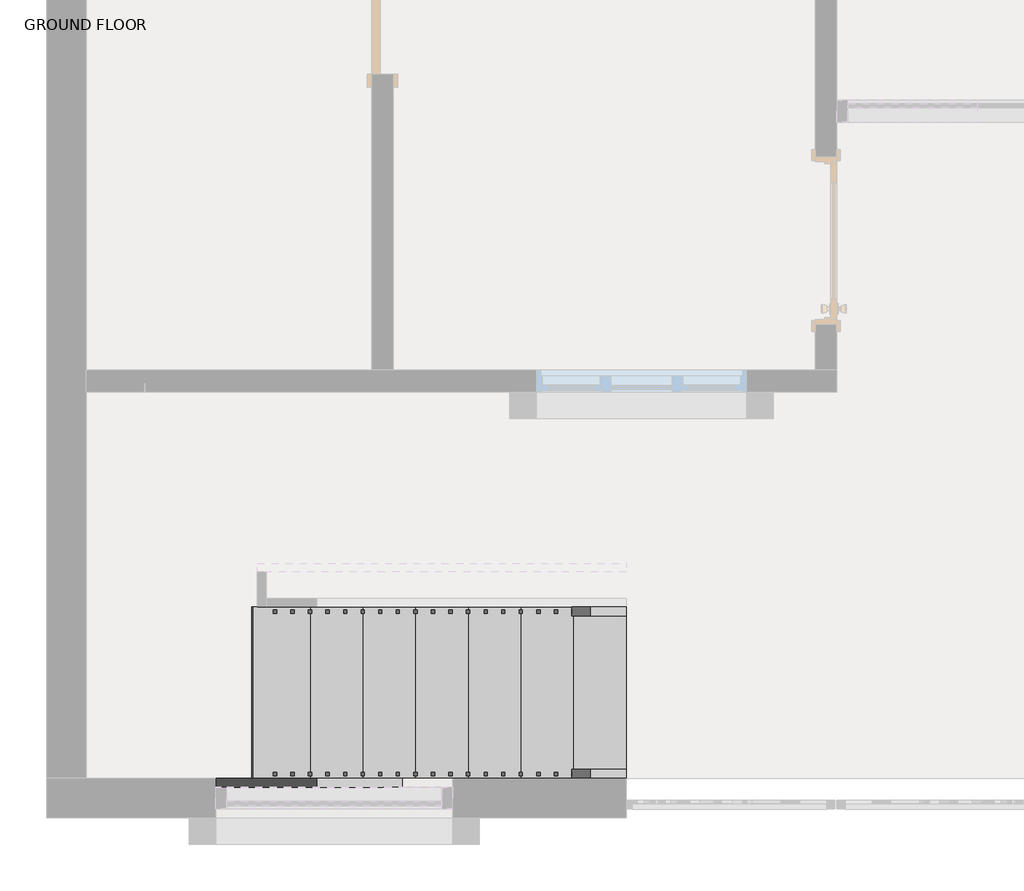
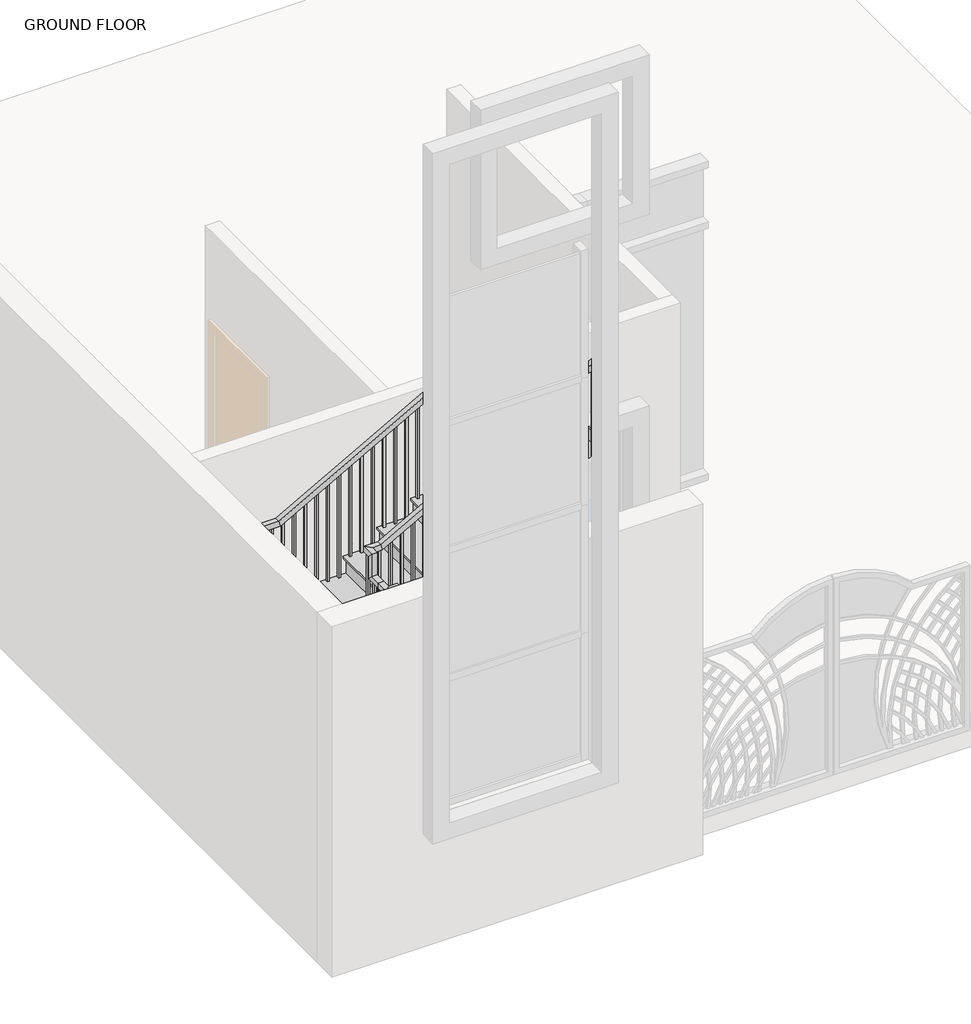
# One storey, part 6 of 7: 2 members, 2 railings, 1 stair flight.
"""IFC4 building model written with IfcOpenShell, lengths in millimetres."""

from ifc_helpers import new_model, si_unit, frame, origin, place, context, project, spatial, polyline, outline, extrude, faceted_brep, transform, mapped, element, save
from components import stair_flight_0a8b780f

model = new_model("IFC4")

# Units and contexts
model_context = context("Model", 3, world=origin())
ifc_project = project(units=[si_unit("LENGTHUNIT", "METRE", prefix="MILLI")], contexts=[model_context])

# Site, building, storey
site = spatial("IfcSite", under=ifc_project)
building = spatial("IfcBuilding", under=site)
storey = spatial("IfcBuildingStorey", under=building, Name="GROUND FLOOR", Elevation=304.8)

# Members
placement = place(None, origin())
element("IfcMember", 1, ObjectType="Stringer - 2\" Width", at=placement, inside=storey, context=model_context, shape_type="SweptSolid", body=[
    extrude(outline(polyline([(304.8, -11636.5023867), (512.3983948, -11636.5023867), (1735.6666667, -13838.3852761), (1735.6666667, -14466.0068895), (304.8, -11890.4468895), (304.8, -11636.5023867)])), frame((0.0, -2807.5499863, 0.0), z_axis=(0.0, 1.0, 0.0), x_axis=(0.0, 0.0, 1.0)), (0.0, 0.0, 1.0), 50.8),
])
element("IfcMember", 2, ObjectType="Stringer - 2\" Width", at=placement, inside=storey, context=model_context, shape_type="SweptSolid", body=[
    extrude(outline(polyline([(-14760.7023867, -2807.5499863), (-14811.5023867, -2807.5499863), (-14811.5023867, -521.5499863), (-14760.7023867, -521.5499863), (-14760.7023867, -2807.5499863)])), frame((0.0, 0.0, 1430.8666667), z_axis=(0.0, 0.0, 1.0), x_axis=(1.0, 0.0, 0.0)), (0.0, 0.0, 1.0), 304.8),
])

# Railings
element("IfcRailing", 3, ObjectType="Handrail - Rectangular", at=placement, inside=storey, context=model_context, shape_type="SolidModel", body=[
    faceted_brep([(-11636.5023867, -1816.9499863, 1388.5333333), (-11636.5023867, -1816.9499863, 1330.420221), (-11636.5023867, -1766.1499863, 1330.420221), (-11636.5023867, -1766.1499863, 1388.5333333), (-13693.9023867, -1816.9499863, 2531.5333333), (-13744.7023867, -1816.9499863, 2501.6424432), (-13744.7023867, -1766.1499863, 2501.6424432), (-13693.9023867, -1766.1499863, 2531.5333333), (-13693.9023867, -1816.9499863, 2573.8666667), (-13744.7023867, -1816.9499863, 2523.0666667), (-13744.7023867, -1766.1499863, 2523.0666667), (-13693.9023867, -1766.1499863, 2573.8666667), (-13820.9023867, -1816.9499863, 2573.8666667), (-13820.9023867, -1816.9499863, 2523.0666667), (-13770.1023867, -1766.1499863, 2523.0666667), (-13770.1023867, -1766.1499863, 2573.8666667), (-13820.9023867, -1689.9499863, 2573.8666667), (-13820.9023867, -1689.9499863, 2523.0666667), (-13770.1023867, -1689.9499863, 2523.0666667), (-13770.1023867, -1689.9499863, 2573.8666667), (-13820.9023867, -1588.3499863, 2573.8666667), (-13820.9023867, -1537.5499863, 2523.0666667), (-13770.1023867, -1537.5499863, 2523.0666667), (-13770.1023867, -1588.3499863, 2573.8666667), (-13820.9023867, -1588.3499863, 2785.5333333), (-13820.9023867, -1537.5499863, 2734.7333333), (-13770.1023867, -1537.5499863, 2734.7333333), (-13770.1023867, -1588.3499863, 2785.5333333), (-13820.9023867, -1461.3499863, 2785.5333333), (-13820.9023867, -1461.3499863, 2734.7333333), (-13770.1023867, -1512.1499863, 2734.7333333), (-13770.1023867, -1512.1499863, 2785.5333333), (-13693.9023867, -1461.3499863, 2785.5333333), (-13680.7387844, -1461.3499863, 2734.7333333), (-13680.7387844, -1512.1499863, 2734.7333333), (-13693.9023867, -1512.1499863, 2785.5333333), (-11636.5023867, -1461.3499863, 3928.5333333), (-11636.5023867, -1512.1499863, 3928.5333333), (-11636.5023867, -1512.1499863, 3870.420221), (-11636.5023867, -1461.3499863, 3870.420221)], [[[0, 1, 2, 3]], [[1, 0, 4, 5]], [[2, 1, 5, 6]], [[3, 2, 6, 7]], [[0, 3, 7, 4]], [[5, 4, 8, 9]], [[6, 5, 9, 10]], [[7, 6, 10, 11]], [[4, 7, 11, 8]], [[9, 8, 12, 13]], [[10, 9, 13, 14]], [[11, 10, 14, 15]], [[8, 11, 15, 12]], [[13, 12, 16, 17]], [[14, 13, 17, 18]], [[15, 14, 18, 19]], [[12, 15, 19, 16]], [[17, 16, 20, 21]], [[18, 17, 21, 22]], [[19, 18, 22, 23]], [[16, 19, 23, 20]], [[21, 20, 24, 25]], [[22, 21, 25, 26]], [[23, 22, 26, 27]], [[20, 23, 27, 24]], [[25, 24, 28, 29]], [[26, 25, 29, 30]], [[27, 26, 30, 31]], [[24, 27, 31, 28]], [[29, 28, 32, 33]], [[30, 29, 33, 34]], [[31, 30, 34, 35]], [[28, 31, 35, 32]], [[36, 37, 38, 39]], [[33, 32, 36, 39]], [[34, 33, 39, 38]], [[35, 34, 38, 37]], [[32, 35, 37, 36]]]),
    extrude(outline(polyline([(3861.6007765, -11652.3773867), (3851.0174432, -11671.4273867), (2844.8, -11671.4273867), (2844.8, -11652.3773867), (3861.6007765, -11652.3773867)])), frame((0.0, -1496.2749863, 0.0), z_axis=(0.0, 1.0, 0.0), x_axis=(0.0, 0.0, 1.0)), (0.0, 0.0, 1.0), 19.05),
    extrude(outline(polyline([(3805.1563321, -11753.9773867), (3794.5729988, -11773.0273867), (2844.8, -11773.0273867), (2844.8, -11753.9773867), (3805.1563321, -11753.9773867)])), frame((0.0, -1496.2749863, 0.0), z_axis=(0.0, 1.0, 0.0), x_axis=(0.0, 0.0, 1.0)), (0.0, 0.0, 1.0), 19.05),
    extrude(outline(polyline([(3748.7118876, -11855.5773867), (3738.1285543, -11874.6273867), (2844.8, -11874.6273867), (2844.8, -11855.5773867), (3748.7118876, -11855.5773867)])), frame((0.0, -1496.2749863, 0.0), z_axis=(0.0, 1.0, 0.0), x_axis=(0.0, 0.0, 1.0)), (0.0, 0.0, 1.0), 19.05),
    extrude(outline(polyline([(3692.2674432, -11957.1773867), (3681.6841099, -11976.2273867), (2675.4666667, -11976.2273867), (2675.4666667, -11957.1773867), (3692.2674432, -11957.1773867)])), frame((0.0, -1496.2749863, 0.0), z_axis=(0.0, 1.0, 0.0), x_axis=(0.0, 0.0, 1.0)), (0.0, 0.0, 1.0), 19.05),
    extrude(outline(polyline([(3635.8229988, -12058.7773867), (3625.2396654, -12077.8273867), (2675.4666667, -12077.8273867), (2675.4666667, -12058.7773867), (3635.8229988, -12058.7773867)])), frame((0.0, -1496.2749863, 0.0), z_axis=(0.0, 1.0, 0.0), x_axis=(0.0, 0.0, 1.0)), (0.0, 0.0, 1.0), 19.05),
    extrude(outline(polyline([(3579.3785543, -12160.3773867), (3568.795221, -12179.4273867), (2675.4666667, -12179.4273867), (2675.4666667, -12160.3773867), (3579.3785543, -12160.3773867)])), frame((0.0, -1496.2749863, 0.0), z_axis=(0.0, 1.0, 0.0), x_axis=(0.0, 0.0, 1.0)), (0.0, 0.0, 1.0), 19.05),
    extrude(outline(polyline([(3522.9341099, -12261.9773867), (3512.3507765, -12281.0273867), (2506.1333333, -12281.0273867), (2506.1333333, -12261.9773867), (3522.9341099, -12261.9773867)])), frame((0.0, -1496.2749863, 0.0), z_axis=(0.0, 1.0, 0.0), x_axis=(0.0, 0.0, 1.0)), (0.0, 0.0, 1.0), 19.05),
    extrude(outline(polyline([(3466.4896654, -12363.5773867), (3455.9063321, -12382.6273867), (2506.1333333, -12382.6273867), (2506.1333333, -12363.5773867), (3466.4896654, -12363.5773867)])), frame((0.0, -1496.2749863, 0.0), z_axis=(0.0, 1.0, 0.0), x_axis=(0.0, 0.0, 1.0)), (0.0, 0.0, 1.0), 19.05),
    extrude(outline(polyline([(3410.045221, -12465.1773867), (3399.4618876, -12484.2273867), (2506.1333333, -12484.2273867), (2506.1333333, -12465.1773867), (3410.045221, -12465.1773867)])), frame((0.0, -1496.2749863, 0.0), z_axis=(0.0, 1.0, 0.0), x_axis=(0.0, 0.0, 1.0)), (0.0, 0.0, 1.0), 19.05),
    extrude(outline(polyline([(3353.6007765, -12566.7773867), (3343.0174432, -12585.8273867), (2336.8, -12585.8273867), (2336.8, -12566.7773867), (3353.6007765, -12566.7773867)])), frame((0.0, -1496.2749863, 0.0), z_axis=(0.0, 1.0, 0.0), x_axis=(0.0, 0.0, 1.0)), (0.0, 0.0, 1.0), 19.05),
    extrude(outline(polyline([(3297.1563321, -12668.3773867), (3286.5729988, -12687.4273867), (2336.8, -12687.4273867), (2336.8, -12668.3773867), (3297.1563321, -12668.3773867)])), frame((0.0, -1496.2749863, 0.0), z_axis=(0.0, 1.0, 0.0), x_axis=(0.0, 0.0, 1.0)), (0.0, 0.0, 1.0), 19.05),
    extrude(outline(polyline([(3240.7118876, -12769.9773867), (3230.1285543, -12789.0273867), (2336.8, -12789.0273867), (2336.8, -12769.9773867), (3240.7118876, -12769.9773867)])), frame((0.0, -1496.2749863, 0.0), z_axis=(0.0, 1.0, 0.0), x_axis=(0.0, 0.0, 1.0)), (0.0, 0.0, 1.0), 19.05),
    extrude(outline(polyline([(3184.2674432, -12871.5773867), (3173.6841099, -12890.6273867), (2167.4666667, -12890.6273867), (2167.4666667, -12871.5773867), (3184.2674432, -12871.5773867)])), frame((0.0, -1496.2749863, 0.0), z_axis=(0.0, 1.0, 0.0), x_axis=(0.0, 0.0, 1.0)), (0.0, 0.0, 1.0), 19.05),
    extrude(outline(polyline([(3127.8229988, -12973.1773867), (3117.2396654, -12992.2273867), (2167.4666667, -12992.2273867), (2167.4666667, -12973.1773867), (3127.8229988, -12973.1773867)])), frame((0.0, -1496.2749863, 0.0), z_axis=(0.0, 1.0, 0.0), x_axis=(0.0, 0.0, 1.0)), (0.0, 0.0, 1.0), 19.05),
    extrude(outline(polyline([(3071.3785543, -13074.7773867), (3060.795221, -13093.8273867), (2167.4666667, -13093.8273867), (2167.4666667, -13074.7773867), (3071.3785543, -13074.7773867)])), frame((0.0, -1496.2749863, 0.0), z_axis=(0.0, 1.0, 0.0), x_axis=(0.0, 0.0, 1.0)), (0.0, 0.0, 1.0), 19.05),
    extrude(outline(polyline([(3014.9341099, -13176.3773867), (3004.3507765, -13195.4273867), (1998.1333333, -13195.4273867), (1998.1333333, -13176.3773867), (3014.9341099, -13176.3773867)])), frame((0.0, -1496.2749863, 0.0), z_axis=(0.0, 1.0, 0.0), x_axis=(0.0, 0.0, 1.0)), (0.0, 0.0, 1.0), 19.05),
    extrude(outline(polyline([(2958.4896654, -13277.9773867), (2947.9063321, -13297.0273867), (1998.1333333, -13297.0273867), (1998.1333333, -13277.9773867), (2958.4896654, -13277.9773867)])), frame((0.0, -1496.2749863, 0.0), z_axis=(0.0, 1.0, 0.0), x_axis=(0.0, 0.0, 1.0)), (0.0, 0.0, 1.0), 19.05),
    extrude(outline(polyline([(2902.045221, -13379.5773867), (2891.4618876, -13398.6273867), (1998.1333333, -13398.6273867), (1998.1333333, -13379.5773867), (2902.045221, -13379.5773867)])), frame((0.0, -1496.2749863, 0.0), z_axis=(0.0, 1.0, 0.0), x_axis=(0.0, 0.0, 1.0)), (0.0, 0.0, 1.0), 19.05),
    extrude(outline(polyline([(2845.6007765, -13481.1773867), (2835.0174432, -13500.2273867), (1828.8, -13500.2273867), (1828.8, -13481.1773867), (2845.6007765, -13481.1773867)])), frame((0.0, -1496.2749863, 0.0), z_axis=(0.0, 1.0, 0.0), x_axis=(0.0, 0.0, 1.0)), (0.0, 0.0, 1.0), 19.05),
    extrude(outline(polyline([(2789.1563321, -13582.7773867), (2778.5729988, -13601.8273867), (1828.8, -13601.8273867), (1828.8, -13582.7773867), (2789.1563321, -13582.7773867)])), frame((0.0, -1496.2749863, 0.0), z_axis=(0.0, 1.0, 0.0), x_axis=(0.0, 0.0, 1.0)), (0.0, 0.0, 1.0), 19.05),
    extrude(outline(polyline([(2732.7118876, -13684.3773867), (2722.1285543, -13703.4273867), (1828.8, -13703.4273867), (1828.8, -13684.3773867), (2732.7118876, -13684.3773867)])), frame((0.0, -1496.2749863, 0.0), z_axis=(0.0, 1.0, 0.0), x_axis=(0.0, 0.0, 1.0)), (0.0, 0.0, 1.0), 19.05),
    extrude(outline(polyline([(-13785.9773867, -1597.8749863), (-13805.0273867, -1597.8749863), (-13805.0273867, -1578.8249863), (-13785.9773867, -1578.8249863), (-13785.9773867, -1597.8749863)])), frame((0.0, 0.0, 1659.4666667), z_axis=(0.0, 0.0, 1.0), x_axis=(1.0, 0.0, 0.0)), (0.0, 0.0, 1.0), 863.6),
    extrude(outline(polyline([(-13785.9773867, -1699.4749863), (-13805.0273867, -1699.4749863), (-13805.0273867, -1680.4249863), (-13785.9773867, -1680.4249863), (-13785.9773867, -1699.4749863)])), frame((0.0, 0.0, 1659.4666667), z_axis=(0.0, 0.0, 1.0), x_axis=(1.0, 0.0, 0.0)), (0.0, 0.0, 1.0), 863.6),
    extrude(outline(polyline([(-13760.5773867, -1782.0249863), (-13760.5773867, -1801.0749863), (-13779.6273867, -1801.0749863), (-13779.6273867, -1782.0249863), (-13760.5773867, -1782.0249863)])), frame((0.0, 0.0, 1659.4666667), z_axis=(0.0, 0.0, 1.0), x_axis=(1.0, 0.0, 0.0)), (0.0, 0.0, 1.0), 863.6),
    extrude(outline(polyline([(2454.0174432, -13658.9773867), (2464.6007765, -13678.0273867), (1490.1333333, -13678.0273867), (1490.1333333, -13658.9773867), (2454.0174432, -13658.9773867)])), frame((0.0, -1801.0749863, 0.0), z_axis=(0.0, 1.0, 0.0), x_axis=(0.0, 0.0, 1.0)), (0.0, 0.0, 1.0), 19.05),
    extrude(outline(polyline([(2397.5729988, -13557.3773867), (2408.1563321, -13576.4273867), (1490.1333333, -13576.4273867), (1490.1333333, -13557.3773867), (2397.5729988, -13557.3773867)])), frame((0.0, -1801.0749863, 0.0), z_axis=(0.0, 1.0, 0.0), x_axis=(0.0, 0.0, 1.0)), (0.0, 0.0, 1.0), 19.05),
    extrude(outline(polyline([(2341.1285543, -13455.7773867), (2351.7118876, -13474.8273867), (1490.1333333, -13474.8273867), (1490.1333333, -13455.7773867), (2341.1285543, -13455.7773867)])), frame((0.0, -1801.0749863, 0.0), z_axis=(0.0, 1.0, 0.0), x_axis=(0.0, 0.0, 1.0)), (0.0, 0.0, 1.0), 19.05),
    extrude(outline(polyline([(2284.6841099, -13354.1773867), (2295.2674432, -13373.2273867), (1320.8, -13373.2273867), (1320.8, -13354.1773867), (2284.6841099, -13354.1773867)])), frame((0.0, -1801.0749863, 0.0), z_axis=(0.0, 1.0, 0.0), x_axis=(0.0, 0.0, 1.0)), (0.0, 0.0, 1.0), 19.05),
    extrude(outline(polyline([(2228.2396654, -13252.5773867), (2238.8229988, -13271.6273867), (1320.8, -13271.6273867), (1320.8, -13252.5773867), (2228.2396654, -13252.5773867)])), frame((0.0, -1801.0749863, 0.0), z_axis=(0.0, 1.0, 0.0), x_axis=(0.0, 0.0, 1.0)), (0.0, 0.0, 1.0), 19.05),
    extrude(outline(polyline([(2171.795221, -13150.9773867), (2182.3785543, -13170.0273867), (1320.8, -13170.0273867), (1320.8, -13150.9773867), (2171.795221, -13150.9773867)])), frame((0.0, -1801.0749863, 0.0), z_axis=(0.0, 1.0, 0.0), x_axis=(0.0, 0.0, 1.0)), (0.0, 0.0, 1.0), 19.05),
    extrude(outline(polyline([(2115.3507765, -13049.3773867), (2125.9341099, -13068.4273867), (1151.4666667, -13068.4273867), (1151.4666667, -13049.3773867), (2115.3507765, -13049.3773867)])), frame((0.0, -1801.0749863, 0.0), z_axis=(0.0, 1.0, 0.0), x_axis=(0.0, 0.0, 1.0)), (0.0, 0.0, 1.0), 19.05),
    extrude(outline(polyline([(2058.9063321, -12947.7773867), (2069.4896654, -12966.8273867), (1151.4666667, -12966.8273867), (1151.4666667, -12947.7773867), (2058.9063321, -12947.7773867)])), frame((0.0, -1801.0749863, 0.0), z_axis=(0.0, 1.0, 0.0), x_axis=(0.0, 0.0, 1.0)), (0.0, 0.0, 1.0), 19.05),
    extrude(outline(polyline([(2002.4618876, -12846.1773867), (2013.045221, -12865.2273867), (1151.4666667, -12865.2273867), (1151.4666667, -12846.1773867), (2002.4618876, -12846.1773867)])), frame((0.0, -1801.0749863, 0.0), z_axis=(0.0, 1.0, 0.0), x_axis=(0.0, 0.0, 1.0)), (0.0, 0.0, 1.0), 19.05),
    extrude(outline(polyline([(1946.0174432, -12744.5773867), (1956.6007765, -12763.6273867), (982.1333333, -12763.6273867), (982.1333333, -12744.5773867), (1946.0174432, -12744.5773867)])), frame((0.0, -1801.0749863, 0.0), z_axis=(0.0, 1.0, 0.0), x_axis=(0.0, 0.0, 1.0)), (0.0, 0.0, 1.0), 19.05),
    extrude(outline(polyline([(1889.5729988, -12642.9773867), (1900.1563321, -12662.0273867), (982.1333333, -12662.0273867), (982.1333333, -12642.9773867), (1889.5729988, -12642.9773867)])), frame((0.0, -1801.0749863, 0.0), z_axis=(0.0, 1.0, 0.0), x_axis=(0.0, 0.0, 1.0)), (0.0, 0.0, 1.0), 19.05),
    extrude(outline(polyline([(1833.1285543, -12541.3773867), (1843.7118876, -12560.4273867), (982.1333333, -12560.4273867), (982.1333333, -12541.3773867), (1833.1285543, -12541.3773867)])), frame((0.0, -1801.0749863, 0.0), z_axis=(0.0, 1.0, 0.0), x_axis=(0.0, 0.0, 1.0)), (0.0, 0.0, 1.0), 19.05),
    extrude(outline(polyline([(1776.6841099, -12439.7773867), (1787.2674432, -12458.8273867), (812.8, -12458.8273867), (812.8, -12439.7773867), (1776.6841099, -12439.7773867)])), frame((0.0, -1801.0749863, 0.0), z_axis=(0.0, 1.0, 0.0), x_axis=(0.0, 0.0, 1.0)), (0.0, 0.0, 1.0), 19.05),
    extrude(outline(polyline([(1720.2396654, -12338.1773867), (1730.8229988, -12357.2273867), (812.8, -12357.2273867), (812.8, -12338.1773867), (1720.2396654, -12338.1773867)])), frame((0.0, -1801.0749863, 0.0), z_axis=(0.0, 1.0, 0.0), x_axis=(0.0, 0.0, 1.0)), (0.0, 0.0, 1.0), 19.05),
    extrude(outline(polyline([(1663.795221, -12236.5773867), (1674.3785543, -12255.6273867), (812.8, -12255.6273867), (812.8, -12236.5773867), (1663.795221, -12236.5773867)])), frame((0.0, -1801.0749863, 0.0), z_axis=(0.0, 1.0, 0.0), x_axis=(0.0, 0.0, 1.0)), (0.0, 0.0, 1.0), 19.05),
    extrude(outline(polyline([(1607.3507765, -12134.9773867), (1617.9341099, -12154.0273867), (643.4666667, -12154.0273867), (643.4666667, -12134.9773867), (1607.3507765, -12134.9773867)])), frame((0.0, -1801.0749863, 0.0), z_axis=(0.0, 1.0, 0.0), x_axis=(0.0, 0.0, 1.0)), (0.0, 0.0, 1.0), 19.05),
    extrude(outline(polyline([(1550.9063321, -12033.3773867), (1561.4896654, -12052.4273867), (643.4666667, -12052.4273867), (643.4666667, -12033.3773867), (1550.9063321, -12033.3773867)])), frame((0.0, -1801.0749863, 0.0), z_axis=(0.0, 1.0, 0.0), x_axis=(0.0, 0.0, 1.0)), (0.0, 0.0, 1.0), 19.05),
    extrude(outline(polyline([(1494.4618876, -11931.7773867), (1505.045221, -11950.8273867), (643.4666667, -11950.8273867), (643.4666667, -11931.7773867), (1494.4618876, -11931.7773867)])), frame((0.0, -1801.0749863, 0.0), z_axis=(0.0, 1.0, 0.0), x_axis=(0.0, 0.0, 1.0)), (0.0, 0.0, 1.0), 19.05),
    extrude(outline(polyline([(1438.0174432, -11830.1773867), (1448.6007765, -11849.2273867), (474.1333333, -11849.2273867), (474.1333333, -11830.1773867), (1438.0174432, -11830.1773867)])), frame((0.0, -1801.0749863, 0.0), z_axis=(0.0, 1.0, 0.0), x_axis=(0.0, 0.0, 1.0)), (0.0, 0.0, 1.0), 19.05),
    extrude(outline(polyline([(1381.5729988, -11728.5773867), (1392.1563321, -11747.6273867), (474.1333333, -11747.6273867), (474.1333333, -11728.5773867), (1381.5729988, -11728.5773867)])), frame((0.0, -1801.0749863, 0.0), z_axis=(0.0, 1.0, 0.0), x_axis=(0.0, 0.0, 1.0)), (0.0, 0.0, 1.0), 19.05),
    extrude(outline(polyline([(-13785.9773867, -1496.2749863), (-13805.0273867, -1496.2749863), (-13805.0273867, -1477.2249863), (-13785.9773867, -1477.2249863), (-13785.9773867, -1496.2749863)])), frame((0.0, 0.0, 1659.4666667), z_axis=(0.0, 0.0, 1.0), x_axis=(1.0, 0.0, 0.0)), (0.0, 0.0, 1.0), 1075.2666667),
    extrude(outline(polyline([(-13785.9773867, -1782.0249863), (-13785.9773867, -1801.0749863), (-13805.0273867, -1801.0749863), (-13805.0273867, -1782.0249863), (-13785.9773867, -1782.0249863)])), frame((0.0, 0.0, 1659.4666667), z_axis=(0.0, 0.0, 1.0), x_axis=(1.0, 0.0, 0.0)), (0.0, 0.0, 1.0), 863.6),
    extrude(outline(polyline([(3870.420221, -11636.5023867), (3859.8368876, -11655.5523867), (2844.8, -11655.5523867), (2844.8, -11636.5023867), (3870.420221, -11636.5023867)])), frame((0.0, -1496.2749863, 0.0), z_axis=(0.0, 1.0, 0.0), x_axis=(0.0, 0.0, 1.0)), (0.0, 0.0, 1.0), 19.05),
    extrude(outline(polyline([(1330.420221, -11636.5023867), (1341.0035543, -11655.5523867), (474.1333333, -11655.5523867), (474.1333333, -11636.5023867), (1330.420221, -11636.5023867)])), frame((0.0, -1801.0749863, 0.0), z_axis=(0.0, 1.0, 0.0), x_axis=(0.0, 0.0, 1.0)), (0.0, 0.0, 1.0), 19.05),
])
element("IfcRailing", 4, ObjectType="Handrail - Rectangular", at=placement, inside=storey, context=model_context, shape_type="SolidModel", body=[
    faceted_brep([(-11636.5023867, -2756.7499863, 1388.5333333), (-11636.5023867, -2756.7499863, 1330.420221), (-11636.5023867, -2705.9499863, 1330.420221), (-11636.5023867, -2705.9499863, 1388.5333333), (-13770.1023867, -2756.7499863, 2573.8666667), (-13783.2659889, -2756.7499863, 2523.0666667), (-13783.2659889, -2705.9499863, 2523.0666667), (-13770.1023867, -2705.9499863, 2573.8666667), (-14760.7023867, -2756.7499863, 2573.8666667), (-14760.7023867, -2756.7499863, 2523.0666667), (-14709.9023867, -2705.9499863, 2523.0666667), (-14709.9023867, -2705.9499863, 2573.8666667), (-14760.7023867, -521.5499863, 2573.8666667), (-14760.7023867, -521.5499863, 2523.0666667), (-14709.9023867, -572.3499863, 2523.0666667), (-14709.9023867, -572.3499863, 2573.8666667), (-14074.9023867, -521.5499863, 2573.8666667), (-14061.7387844, -521.5499863, 2523.0666667), (-14061.7387844, -572.3499863, 2523.0666667), (-14074.9023867, -572.3499863, 2573.8666667), (-11636.5023867, -521.5499863, 3928.5333333), (-11636.5023867, -572.3499863, 3928.5333333), (-11636.5023867, -572.3499863, 3870.420221), (-11636.5023867, -521.5499863, 3870.420221)], [[[0, 1, 2, 3]], [[1, 0, 4, 5]], [[2, 1, 5, 6]], [[3, 2, 6, 7]], [[0, 3, 7, 4]], [[5, 4, 8, 9]], [[6, 5, 9, 10]], [[7, 6, 10, 11]], [[4, 7, 11, 8]], [[9, 8, 12, 13]], [[10, 9, 13, 14]], [[11, 10, 14, 15]], [[8, 11, 15, 12]], [[13, 12, 16, 17]], [[14, 13, 17, 18]], [[15, 14, 18, 19]], [[12, 15, 19, 16]], [[20, 21, 22, 23]], [[17, 16, 20, 23]], [[18, 17, 23, 22]], [[19, 18, 22, 21]], [[16, 19, 21, 20]]]),
    extrude(outline(polyline([(3836.9063321, -11696.8273867), (2844.8, -11696.8273867), (2844.8, -11677.7773867), (3847.4896654, -11677.7773867), (3836.9063321, -11696.8273867)])), frame((0.0, -556.4749863, 0.0), z_axis=(0.0, 1.0, 0.0), x_axis=(0.0, 0.0, 1.0)), (0.0, 0.0, 1.0), 19.05),
    extrude(outline(polyline([(3780.4618876, -11798.4273867), (2844.8, -11798.4273867), (2844.8, -11779.3773867), (3791.045221, -11779.3773867), (3780.4618876, -11798.4273867)])), frame((0.0, -556.4749863, 0.0), z_axis=(0.0, 1.0, 0.0), x_axis=(0.0, 0.0, 1.0)), (0.0, 0.0, 1.0), 19.05),
    extrude(outline(polyline([(3724.0174432, -11900.0273867), (2844.8, -11900.0273867), (2844.8, -11880.9773867), (3734.6007765, -11880.9773867), (3724.0174432, -11900.0273867)])), frame((0.0, -556.4749863, 0.0), z_axis=(0.0, 1.0, 0.0), x_axis=(0.0, 0.0, 1.0)), (0.0, 0.0, 1.0), 19.05),
    extrude(outline(polyline([(3667.5729988, -12001.6273867), (2675.4666667, -12001.6273867), (2675.4666667, -11982.5773867), (3678.1563321, -11982.5773867), (3667.5729988, -12001.6273867)])), frame((0.0, -556.4749863, 0.0), z_axis=(0.0, 1.0, 0.0), x_axis=(0.0, 0.0, 1.0)), (0.0, 0.0, 1.0), 19.05),
    extrude(outline(polyline([(3611.1285543, -12103.2273867), (2675.4666667, -12103.2273867), (2675.4666667, -12084.1773867), (3621.7118876, -12084.1773867), (3611.1285543, -12103.2273867)])), frame((0.0, -556.4749863, 0.0), z_axis=(0.0, 1.0, 0.0), x_axis=(0.0, 0.0, 1.0)), (0.0, 0.0, 1.0), 19.05),
    extrude(outline(polyline([(3554.6841099, -12204.8273867), (2675.4666667, -12204.8273867), (2675.4666667, -12185.7773867), (3565.2674432, -12185.7773867), (3554.6841099, -12204.8273867)])), frame((0.0, -556.4749863, 0.0), z_axis=(0.0, 1.0, 0.0), x_axis=(0.0, 0.0, 1.0)), (0.0, 0.0, 1.0), 19.05),
    extrude(outline(polyline([(3498.2396654, -12306.4273867), (2506.1333333, -12306.4273867), (2506.1333333, -12287.3773867), (3508.8229988, -12287.3773867), (3498.2396654, -12306.4273867)])), frame((0.0, -556.4749863, 0.0), z_axis=(0.0, 1.0, 0.0), x_axis=(0.0, 0.0, 1.0)), (0.0, 0.0, 1.0), 19.05),
    extrude(outline(polyline([(3441.795221, -12408.0273867), (2506.1333333, -12408.0273867), (2506.1333333, -12388.9773867), (3452.3785543, -12388.9773867), (3441.795221, -12408.0273867)])), frame((0.0, -556.4749863, 0.0), z_axis=(0.0, 1.0, 0.0), x_axis=(0.0, 0.0, 1.0)), (0.0, 0.0, 1.0), 19.05),
    extrude(outline(polyline([(3385.3507765, -12509.6273867), (2506.1333333, -12509.6273867), (2506.1333333, -12490.5773867), (3395.9341099, -12490.5773867), (3385.3507765, -12509.6273867)])), frame((0.0, -556.4749863, 0.0), z_axis=(0.0, 1.0, 0.0), x_axis=(0.0, 0.0, 1.0)), (0.0, 0.0, 1.0), 19.05),
    extrude(outline(polyline([(3328.9063321, -12611.2273867), (2336.8, -12611.2273867), (2336.8, -12592.1773867), (3339.4896654, -12592.1773867), (3328.9063321, -12611.2273867)])), frame((0.0, -556.4749863, 0.0), z_axis=(0.0, 1.0, 0.0), x_axis=(0.0, 0.0, 1.0)), (0.0, 0.0, 1.0), 19.05),
    extrude(outline(polyline([(3272.4618876, -12712.8273867), (2336.8, -12712.8273867), (2336.8, -12693.7773867), (3283.045221, -12693.7773867), (3272.4618876, -12712.8273867)])), frame((0.0, -556.4749863, 0.0), z_axis=(0.0, 1.0, 0.0), x_axis=(0.0, 0.0, 1.0)), (0.0, 0.0, 1.0), 19.05),
    extrude(outline(polyline([(3216.0174432, -12814.4273867), (2336.8, -12814.4273867), (2336.8, -12795.3773867), (3226.6007765, -12795.3773867), (3216.0174432, -12814.4273867)])), frame((0.0, -556.4749863, 0.0), z_axis=(0.0, 1.0, 0.0), x_axis=(0.0, 0.0, 1.0)), (0.0, 0.0, 1.0), 19.05),
    extrude(outline(polyline([(3159.5729988, -12916.0273867), (2167.4666667, -12916.0273867), (2167.4666667, -12896.9773867), (3170.1563321, -12896.9773867), (3159.5729988, -12916.0273867)])), frame((0.0, -556.4749863, 0.0), z_axis=(0.0, 1.0, 0.0), x_axis=(0.0, 0.0, 1.0)), (0.0, 0.0, 1.0), 19.05),
    extrude(outline(polyline([(3103.1285543, -13017.6273867), (2167.4666667, -13017.6273867), (2167.4666667, -12998.5773867), (3113.7118876, -12998.5773867), (3103.1285543, -13017.6273867)])), frame((0.0, -556.4749863, 0.0), z_axis=(0.0, 1.0, 0.0), x_axis=(0.0, 0.0, 1.0)), (0.0, 0.0, 1.0), 19.05),
    extrude(outline(polyline([(3046.6841099, -13119.2273867), (2167.4666667, -13119.2273867), (2167.4666667, -13100.1773867), (3057.2674432, -13100.1773867), (3046.6841099, -13119.2273867)])), frame((0.0, -556.4749863, 0.0), z_axis=(0.0, 1.0, 0.0), x_axis=(0.0, 0.0, 1.0)), (0.0, 0.0, 1.0), 19.05),
    extrude(outline(polyline([(2990.2396654, -13220.8273867), (1998.1333333, -13220.8273867), (1998.1333333, -13201.7773867), (3000.8229988, -13201.7773867), (2990.2396654, -13220.8273867)])), frame((0.0, -556.4749863, 0.0), z_axis=(0.0, 1.0, 0.0), x_axis=(0.0, 0.0, 1.0)), (0.0, 0.0, 1.0), 19.05),
    extrude(outline(polyline([(2933.795221, -13322.4273867), (1998.1333333, -13322.4273867), (1998.1333333, -13303.3773867), (2944.3785543, -13303.3773867), (2933.795221, -13322.4273867)])), frame((0.0, -556.4749863, 0.0), z_axis=(0.0, 1.0, 0.0), x_axis=(0.0, 0.0, 1.0)), (0.0, 0.0, 1.0), 19.05),
    extrude(outline(polyline([(2877.3507765, -13424.0273867), (1998.1333333, -13424.0273867), (1998.1333333, -13404.9773867), (2887.9341099, -13404.9773867), (2877.3507765, -13424.0273867)])), frame((0.0, -556.4749863, 0.0), z_axis=(0.0, 1.0, 0.0), x_axis=(0.0, 0.0, 1.0)), (0.0, 0.0, 1.0), 19.05),
    extrude(outline(polyline([(2820.9063321, -13525.6273867), (1828.8, -13525.6273867), (1828.8, -13506.5773867), (2831.4896654, -13506.5773867), (2820.9063321, -13525.6273867)])), frame((0.0, -556.4749863, 0.0), z_axis=(0.0, 1.0, 0.0), x_axis=(0.0, 0.0, 1.0)), (0.0, 0.0, 1.0), 19.05),
    extrude(outline(polyline([(2764.4618876, -13627.2273867), (1828.8, -13627.2273867), (1828.8, -13608.1773867), (2775.045221, -13608.1773867), (2764.4618876, -13627.2273867)])), frame((0.0, -556.4749863, 0.0), z_axis=(0.0, 1.0, 0.0), x_axis=(0.0, 0.0, 1.0)), (0.0, 0.0, 1.0), 19.05),
    extrude(outline(polyline([(2708.0174432, -13728.8273867), (1828.8, -13728.8273867), (1828.8, -13709.7773867), (2718.6007765, -13709.7773867), (2708.0174432, -13728.8273867)])), frame((0.0, -556.4749863, 0.0), z_axis=(0.0, 1.0, 0.0), x_axis=(0.0, 0.0, 1.0)), (0.0, 0.0, 1.0), 19.05),
    extrude(outline(polyline([(2651.5729988, -13830.4273867), (1659.4666667, -13830.4273867), (1659.4666667, -13811.3773867), (2662.1563321, -13811.3773867), (2651.5729988, -13830.4273867)])), frame((0.0, -556.4749863, 0.0), z_axis=(0.0, 1.0, 0.0), x_axis=(0.0, 0.0, 1.0)), (0.0, 0.0, 1.0), 19.05),
    extrude(outline(polyline([(2595.1285543, -13932.0273867), (1659.4666667, -13932.0273867), (1659.4666667, -13912.9773867), (2605.7118876, -13912.9773867), (2595.1285543, -13932.0273867)])), frame((0.0, -556.4749863, 0.0), z_axis=(0.0, 1.0, 0.0), x_axis=(0.0, 0.0, 1.0)), (0.0, 0.0, 1.0), 19.05),
    extrude(outline(polyline([(2538.6841099, -14033.6273867), (1659.4666667, -14033.6273867), (1659.4666667, -14014.5773867), (2549.2674432, -14014.5773867), (2538.6841099, -14033.6273867)])), frame((0.0, -556.4749863, 0.0), z_axis=(0.0, 1.0, 0.0), x_axis=(0.0, 0.0, 1.0)), (0.0, 0.0, 1.0), 19.05),
    extrude(outline(polyline([(-14135.2273867, -537.4249863), (-14116.1773867, -537.4249863), (-14116.1773867, -556.4749863), (-14135.2273867, -556.4749863), (-14135.2273867, -537.4249863)])), frame((0.0, 0.0, 1659.4666667), z_axis=(0.0, 0.0, 1.0), x_axis=(1.0, 0.0, 0.0)), (0.0, 0.0, 1.0), 863.6),
    extrude(outline(polyline([(-14236.8273867, -537.4249863), (-14217.7773867, -537.4249863), (-14217.7773867, -556.4749863), (-14236.8273867, -556.4749863), (-14236.8273867, -537.4249863)])), frame((0.0, 0.0, 1659.4666667), z_axis=(0.0, 0.0, 1.0), x_axis=(1.0, 0.0, 0.0)), (0.0, 0.0, 1.0), 863.6),
    extrude(outline(polyline([(-14338.4273867, -537.4249863), (-14319.3773867, -537.4249863), (-14319.3773867, -556.4749863), (-14338.4273867, -556.4749863), (-14338.4273867, -537.4249863)])), frame((0.0, 0.0, 1659.4666667), z_axis=(0.0, 0.0, 1.0), x_axis=(1.0, 0.0, 0.0)), (0.0, 0.0, 1.0), 863.6),
    extrude(outline(polyline([(-14440.0273867, -537.4249863), (-14420.9773867, -537.4249863), (-14420.9773867, -556.4749863), (-14440.0273867, -556.4749863), (-14440.0273867, -537.4249863)])), frame((0.0, 0.0, 1659.4666667), z_axis=(0.0, 0.0, 1.0), x_axis=(1.0, 0.0, 0.0)), (0.0, 0.0, 1.0), 863.6),
    extrude(outline(polyline([(-14541.6273867, -537.4249863), (-14522.5773867, -537.4249863), (-14522.5773867, -556.4749863), (-14541.6273867, -556.4749863), (-14541.6273867, -537.4249863)])), frame((0.0, 0.0, 1659.4666667), z_axis=(0.0, 0.0, 1.0), x_axis=(1.0, 0.0, 0.0)), (0.0, 0.0, 1.0), 863.6),
    extrude(outline(polyline([(-14643.2273867, -537.4249863), (-14624.1773867, -537.4249863), (-14624.1773867, -556.4749863), (-14643.2273867, -556.4749863), (-14643.2273867, -537.4249863)])), frame((0.0, 0.0, 1659.4666667), z_axis=(0.0, 0.0, 1.0), x_axis=(1.0, 0.0, 0.0)), (0.0, 0.0, 1.0), 863.6),
    extrude(outline(polyline([(-14744.8273867, -607.2749863), (-14744.8273867, -588.2249863), (-14725.7773867, -588.2249863), (-14725.7773867, -607.2749863), (-14744.8273867, -607.2749863)])), frame((0.0, 0.0, 1659.4666667), z_axis=(0.0, 0.0, 1.0), x_axis=(1.0, 0.0, 0.0)), (0.0, 0.0, 1.0), 863.6),
    extrude(outline(polyline([(-14744.8273867, -708.8749863), (-14744.8273867, -689.8249863), (-14725.7773867, -689.8249863), (-14725.7773867, -708.8749863), (-14744.8273867, -708.8749863)])), frame((0.0, 0.0, 1659.4666667), z_axis=(0.0, 0.0, 1.0), x_axis=(1.0, 0.0, 0.0)), (0.0, 0.0, 1.0), 863.6),
    extrude(outline(polyline([(-14744.8273867, -810.4749863), (-14744.8273867, -791.4249863), (-14725.7773867, -791.4249863), (-14725.7773867, -810.4749863), (-14744.8273867, -810.4749863)])), frame((0.0, 0.0, 1659.4666667), z_axis=(0.0, 0.0, 1.0), x_axis=(1.0, 0.0, 0.0)), (0.0, 0.0, 1.0), 863.6),
    extrude(outline(polyline([(-14744.8273867, -912.0749863), (-14744.8273867, -893.0249863), (-14725.7773867, -893.0249863), (-14725.7773867, -912.0749863), (-14744.8273867, -912.0749863)])), frame((0.0, 0.0, 1659.4666667), z_axis=(0.0, 0.0, 1.0), x_axis=(1.0, 0.0, 0.0)), (0.0, 0.0, 1.0), 863.6),
    extrude(outline(polyline([(-14744.8273867, -1013.6749863), (-14744.8273867, -994.6249863), (-14725.7773867, -994.6249863), (-14725.7773867, -1013.6749863), (-14744.8273867, -1013.6749863)])), frame((0.0, 0.0, 1659.4666667), z_axis=(0.0, 0.0, 1.0), x_axis=(1.0, 0.0, 0.0)), (0.0, 0.0, 1.0), 863.6),
    extrude(outline(polyline([(-14744.8273867, -1115.2749863), (-14744.8273867, -1096.2249863), (-14725.7773867, -1096.2249863), (-14725.7773867, -1115.2749863), (-14744.8273867, -1115.2749863)])), frame((0.0, 0.0, 1659.4666667), z_axis=(0.0, 0.0, 1.0), x_axis=(1.0, 0.0, 0.0)), (0.0, 0.0, 1.0), 863.6),
    extrude(outline(polyline([(-14744.8273867, -1216.8749863), (-14744.8273867, -1197.8249863), (-14725.7773867, -1197.8249863), (-14725.7773867, -1216.8749863), (-14744.8273867, -1216.8749863)])), frame((0.0, 0.0, 1659.4666667), z_axis=(0.0, 0.0, 1.0), x_axis=(1.0, 0.0, 0.0)), (0.0, 0.0, 1.0), 863.6),
    extrude(outline(polyline([(-14744.8273867, -1318.4749863), (-14744.8273867, -1299.4249863), (-14725.7773867, -1299.4249863), (-14725.7773867, -1318.4749863), (-14744.8273867, -1318.4749863)])), frame((0.0, 0.0, 1659.4666667), z_axis=(0.0, 0.0, 1.0), x_axis=(1.0, 0.0, 0.0)), (0.0, 0.0, 1.0), 863.6),
    extrude(outline(polyline([(-14744.8273867, -1420.0749863), (-14744.8273867, -1401.0249863), (-14725.7773867, -1401.0249863), (-14725.7773867, -1420.0749863), (-14744.8273867, -1420.0749863)])), frame((0.0, 0.0, 1659.4666667), z_axis=(0.0, 0.0, 1.0), x_axis=(1.0, 0.0, 0.0)), (0.0, 0.0, 1.0), 863.6),
    extrude(outline(polyline([(-14744.8273867, -1521.6749863), (-14744.8273867, -1502.6249863), (-14725.7773867, -1502.6249863), (-14725.7773867, -1521.6749863), (-14744.8273867, -1521.6749863)])), frame((0.0, 0.0, 1659.4666667), z_axis=(0.0, 0.0, 1.0), x_axis=(1.0, 0.0, 0.0)), (0.0, 0.0, 1.0), 863.6),
    extrude(outline(polyline([(-14744.8273867, -1623.2749863), (-14744.8273867, -1604.2249863), (-14725.7773867, -1604.2249863), (-14725.7773867, -1623.2749863), (-14744.8273867, -1623.2749863)])), frame((0.0, 0.0, 1659.4666667), z_axis=(0.0, 0.0, 1.0), x_axis=(1.0, 0.0, 0.0)), (0.0, 0.0, 1.0), 863.6),
    extrude(outline(polyline([(-14744.8273867, -1724.8749863), (-14744.8273867, -1705.8249863), (-14725.7773867, -1705.8249863), (-14725.7773867, -1724.8749863), (-14744.8273867, -1724.8749863)])), frame((0.0, 0.0, 1659.4666667), z_axis=(0.0, 0.0, 1.0), x_axis=(1.0, 0.0, 0.0)), (0.0, 0.0, 1.0), 863.6),
    extrude(outline(polyline([(-14744.8273867, -1826.4749863), (-14744.8273867, -1807.4249863), (-14725.7773867, -1807.4249863), (-14725.7773867, -1826.4749863), (-14744.8273867, -1826.4749863)])), frame((0.0, 0.0, 1659.4666667), z_axis=(0.0, 0.0, 1.0), x_axis=(1.0, 0.0, 0.0)), (0.0, 0.0, 1.0), 863.6),
    extrude(outline(polyline([(-14744.8273867, -1928.0749863), (-14744.8273867, -1909.0249863), (-14725.7773867, -1909.0249863), (-14725.7773867, -1928.0749863), (-14744.8273867, -1928.0749863)])), frame((0.0, 0.0, 1659.4666667), z_axis=(0.0, 0.0, 1.0), x_axis=(1.0, 0.0, 0.0)), (0.0, 0.0, 1.0), 863.6),
    extrude(outline(polyline([(-14744.8273867, -2029.6749863), (-14744.8273867, -2010.6249863), (-14725.7773867, -2010.6249863), (-14725.7773867, -2029.6749863), (-14744.8273867, -2029.6749863)])), frame((0.0, 0.0, 1659.4666667), z_axis=(0.0, 0.0, 1.0), x_axis=(1.0, 0.0, 0.0)), (0.0, 0.0, 1.0), 863.6),
    extrude(outline(polyline([(-14744.8273867, -2131.2749863), (-14744.8273867, -2112.2249863), (-14725.7773867, -2112.2249863), (-14725.7773867, -2131.2749863), (-14744.8273867, -2131.2749863)])), frame((0.0, 0.0, 1659.4666667), z_axis=(0.0, 0.0, 1.0), x_axis=(1.0, 0.0, 0.0)), (0.0, 0.0, 1.0), 863.6),
    extrude(outline(polyline([(-14744.8273867, -2232.8749863), (-14744.8273867, -2213.8249863), (-14725.7773867, -2213.8249863), (-14725.7773867, -2232.8749863), (-14744.8273867, -2232.8749863)])), frame((0.0, 0.0, 1659.4666667), z_axis=(0.0, 0.0, 1.0), x_axis=(1.0, 0.0, 0.0)), (0.0, 0.0, 1.0), 863.6),
    extrude(outline(polyline([(-14744.8273867, -2334.4749863), (-14744.8273867, -2315.4249863), (-14725.7773867, -2315.4249863), (-14725.7773867, -2334.4749863), (-14744.8273867, -2334.4749863)])), frame((0.0, 0.0, 1659.4666667), z_axis=(0.0, 0.0, 1.0), x_axis=(1.0, 0.0, 0.0)), (0.0, 0.0, 1.0), 863.6),
    extrude(outline(polyline([(-14744.8273867, -2436.0749863), (-14744.8273867, -2417.0249863), (-14725.7773867, -2417.0249863), (-14725.7773867, -2436.0749863), (-14744.8273867, -2436.0749863)])), frame((0.0, 0.0, 1659.4666667), z_axis=(0.0, 0.0, 1.0), x_axis=(1.0, 0.0, 0.0)), (0.0, 0.0, 1.0), 863.6),
    extrude(outline(polyline([(-14744.8273867, -2537.6749863), (-14744.8273867, -2518.6249863), (-14725.7773867, -2518.6249863), (-14725.7773867, -2537.6749863), (-14744.8273867, -2537.6749863)])), frame((0.0, 0.0, 1659.4666667), z_axis=(0.0, 0.0, 1.0), x_axis=(1.0, 0.0, 0.0)), (0.0, 0.0, 1.0), 863.6),
    extrude(outline(polyline([(-14744.8273867, -2639.2749863), (-14744.8273867, -2620.2249863), (-14725.7773867, -2620.2249863), (-14725.7773867, -2639.2749863), (-14744.8273867, -2639.2749863)])), frame((0.0, 0.0, 1659.4666667), z_axis=(0.0, 0.0, 1.0), x_axis=(1.0, 0.0, 0.0)), (0.0, 0.0, 1.0), 863.6),
    extrude(outline(polyline([(-14674.9773867, -2740.8749863), (-14694.0273867, -2740.8749863), (-14694.0273867, -2721.8249863), (-14674.9773867, -2721.8249863), (-14674.9773867, -2740.8749863)])), frame((0.0, 0.0, 1659.4666667), z_axis=(0.0, 0.0, 1.0), x_axis=(1.0, 0.0, 0.0)), (0.0, 0.0, 1.0), 863.6),
    extrude(outline(polyline([(-14573.3773867, -2740.8749863), (-14592.4273867, -2740.8749863), (-14592.4273867, -2721.8249863), (-14573.3773867, -2721.8249863), (-14573.3773867, -2740.8749863)])), frame((0.0, 0.0, 1659.4666667), z_axis=(0.0, 0.0, 1.0), x_axis=(1.0, 0.0, 0.0)), (0.0, 0.0, 1.0), 863.6),
    extrude(outline(polyline([(-14471.7773867, -2740.8749863), (-14490.8273867, -2740.8749863), (-14490.8273867, -2721.8249863), (-14471.7773867, -2721.8249863), (-14471.7773867, -2740.8749863)])), frame((0.0, 0.0, 1659.4666667), z_axis=(0.0, 0.0, 1.0), x_axis=(1.0, 0.0, 0.0)), (0.0, 0.0, 1.0), 863.6),
    extrude(outline(polyline([(-14370.1773867, -2740.8749863), (-14389.2273867, -2740.8749863), (-14389.2273867, -2721.8249863), (-14370.1773867, -2721.8249863), (-14370.1773867, -2740.8749863)])), frame((0.0, 0.0, 1659.4666667), z_axis=(0.0, 0.0, 1.0), x_axis=(1.0, 0.0, 0.0)), (0.0, 0.0, 1.0), 863.6),
    extrude(outline(polyline([(-14268.5773867, -2740.8749863), (-14287.6273867, -2740.8749863), (-14287.6273867, -2721.8249863), (-14268.5773867, -2721.8249863), (-14268.5773867, -2740.8749863)])), frame((0.0, 0.0, 1659.4666667), z_axis=(0.0, 0.0, 1.0), x_axis=(1.0, 0.0, 0.0)), (0.0, 0.0, 1.0), 863.6),
    extrude(outline(polyline([(-14166.9773867, -2740.8749863), (-14186.0273867, -2740.8749863), (-14186.0273867, -2721.8249863), (-14166.9773867, -2721.8249863), (-14166.9773867, -2740.8749863)])), frame((0.0, 0.0, 1659.4666667), z_axis=(0.0, 0.0, 1.0), x_axis=(1.0, 0.0, 0.0)), (0.0, 0.0, 1.0), 863.6),
    extrude(outline(polyline([(-14065.3773867, -2740.8749863), (-14084.4273867, -2740.8749863), (-14084.4273867, -2721.8249863), (-14065.3773867, -2721.8249863), (-14065.3773867, -2740.8749863)])), frame((0.0, 0.0, 1659.4666667), z_axis=(0.0, 0.0, 1.0), x_axis=(1.0, 0.0, 0.0)), (0.0, 0.0, 1.0), 863.6),
    extrude(outline(polyline([(-13963.7773867, -2740.8749863), (-13982.8273867, -2740.8749863), (-13982.8273867, -2721.8249863), (-13963.7773867, -2721.8249863), (-13963.7773867, -2740.8749863)])), frame((0.0, 0.0, 1659.4666667), z_axis=(0.0, 0.0, 1.0), x_axis=(1.0, 0.0, 0.0)), (0.0, 0.0, 1.0), 863.6),
    extrude(outline(polyline([(-13862.1773867, -2740.8749863), (-13881.2273867, -2740.8749863), (-13881.2273867, -2721.8249863), (-13862.1773867, -2721.8249863), (-13862.1773867, -2740.8749863)])), frame((0.0, 0.0, 1659.4666667), z_axis=(0.0, 0.0, 1.0), x_axis=(1.0, 0.0, 0.0)), (0.0, 0.0, 1.0), 863.6),
    extrude(outline(polyline([(2521.045221, -13779.6273867), (1659.4666667, -13779.6273867), (1659.4666667, -13760.5773867), (2510.4618876, -13760.5773867), (2521.045221, -13779.6273867)])), frame((0.0, -2740.8749863, 0.0), z_axis=(0.0, 1.0, 0.0), x_axis=(0.0, 0.0, 1.0)), (0.0, 0.0, 1.0), 19.05),
    extrude(outline(polyline([(2464.6007765, -13678.0273867), (1490.1333333, -13678.0273867), (1490.1333333, -13658.9773867), (2454.0174432, -13658.9773867), (2464.6007765, -13678.0273867)])), frame((0.0, -2740.8749863, 0.0), z_axis=(0.0, 1.0, 0.0), x_axis=(0.0, 0.0, 1.0)), (0.0, 0.0, 1.0), 19.05),
    extrude(outline(polyline([(2408.1563321, -13576.4273867), (1490.1333333, -13576.4273867), (1490.1333333, -13557.3773867), (2397.5729988, -13557.3773867), (2408.1563321, -13576.4273867)])), frame((0.0, -2740.8749863, 0.0), z_axis=(0.0, 1.0, 0.0), x_axis=(0.0, 0.0, 1.0)), (0.0, 0.0, 1.0), 19.05),
    extrude(outline(polyline([(2351.7118876, -13474.8273867), (1490.1333333, -13474.8273867), (1490.1333333, -13455.7773867), (2341.1285543, -13455.7773867), (2351.7118876, -13474.8273867)])), frame((0.0, -2740.8749863, 0.0), z_axis=(0.0, 1.0, 0.0), x_axis=(0.0, 0.0, 1.0)), (0.0, 0.0, 1.0), 19.05),
    extrude(outline(polyline([(2295.2674432, -13373.2273867), (1320.8, -13373.2273867), (1320.8, -13354.1773867), (2284.6841099, -13354.1773867), (2295.2674432, -13373.2273867)])), frame((0.0, -2740.8749863, 0.0), z_axis=(0.0, 1.0, 0.0), x_axis=(0.0, 0.0, 1.0)), (0.0, 0.0, 1.0), 19.05),
    extrude(outline(polyline([(2238.8229988, -13271.6273867), (1320.8, -13271.6273867), (1320.8, -13252.5773867), (2228.2396654, -13252.5773867), (2238.8229988, -13271.6273867)])), frame((0.0, -2740.8749863, 0.0), z_axis=(0.0, 1.0, 0.0), x_axis=(0.0, 0.0, 1.0)), (0.0, 0.0, 1.0), 19.05),
    extrude(outline(polyline([(2182.3785543, -13170.0273867), (1320.8, -13170.0273867), (1320.8, -13150.9773867), (2171.795221, -13150.9773867), (2182.3785543, -13170.0273867)])), frame((0.0, -2740.8749863, 0.0), z_axis=(0.0, 1.0, 0.0), x_axis=(0.0, 0.0, 1.0)), (0.0, 0.0, 1.0), 19.05),
    extrude(outline(polyline([(2125.9341099, -13068.4273867), (1151.4666667, -13068.4273867), (1151.4666667, -13049.3773867), (2115.3507765, -13049.3773867), (2125.9341099, -13068.4273867)])), frame((0.0, -2740.8749863, 0.0), z_axis=(0.0, 1.0, 0.0), x_axis=(0.0, 0.0, 1.0)), (0.0, 0.0, 1.0), 19.05),
    extrude(outline(polyline([(2069.4896654, -12966.8273867), (1151.4666667, -12966.8273867), (1151.4666667, -12947.7773867), (2058.9063321, -12947.7773867), (2069.4896654, -12966.8273867)])), frame((0.0, -2740.8749863, 0.0), z_axis=(0.0, 1.0, 0.0), x_axis=(0.0, 0.0, 1.0)), (0.0, 0.0, 1.0), 19.05),
    extrude(outline(polyline([(2013.045221, -12865.2273867), (1151.4666667, -12865.2273867), (1151.4666667, -12846.1773867), (2002.4618876, -12846.1773867), (2013.045221, -12865.2273867)])), frame((0.0, -2740.8749863, 0.0), z_axis=(0.0, 1.0, 0.0), x_axis=(0.0, 0.0, 1.0)), (0.0, 0.0, 1.0), 19.05),
    extrude(outline(polyline([(1956.6007765, -12763.6273867), (982.1333333, -12763.6273867), (982.1333333, -12744.5773867), (1946.0174432, -12744.5773867), (1956.6007765, -12763.6273867)])), frame((0.0, -2740.8749863, 0.0), z_axis=(0.0, 1.0, 0.0), x_axis=(0.0, 0.0, 1.0)), (0.0, 0.0, 1.0), 19.05),
    extrude(outline(polyline([(1900.1563321, -12662.0273867), (982.1333333, -12662.0273867), (982.1333333, -12642.9773867), (1889.5729988, -12642.9773867), (1900.1563321, -12662.0273867)])), frame((0.0, -2740.8749863, 0.0), z_axis=(0.0, 1.0, 0.0), x_axis=(0.0, 0.0, 1.0)), (0.0, 0.0, 1.0), 19.05),
    extrude(outline(polyline([(1843.7118876, -12560.4273867), (982.1333333, -12560.4273867), (982.1333333, -12541.3773867), (1833.1285543, -12541.3773867), (1843.7118876, -12560.4273867)])), frame((0.0, -2740.8749863, 0.0), z_axis=(0.0, 1.0, 0.0), x_axis=(0.0, 0.0, 1.0)), (0.0, 0.0, 1.0), 19.05),
    extrude(outline(polyline([(1787.2674432, -12458.8273867), (812.8, -12458.8273867), (812.8, -12439.7773867), (1776.6841099, -12439.7773867), (1787.2674432, -12458.8273867)])), frame((0.0, -2740.8749863, 0.0), z_axis=(0.0, 1.0, 0.0), x_axis=(0.0, 0.0, 1.0)), (0.0, 0.0, 1.0), 19.05),
    extrude(outline(polyline([(1730.8229988, -12357.2273867), (812.8, -12357.2273867), (812.8, -12338.1773867), (1720.2396654, -12338.1773867), (1730.8229988, -12357.2273867)])), frame((0.0, -2740.8749863, 0.0), z_axis=(0.0, 1.0, 0.0), x_axis=(0.0, 0.0, 1.0)), (0.0, 0.0, 1.0), 19.05),
    extrude(outline(polyline([(1674.3785543, -12255.6273867), (812.8, -12255.6273867), (812.8, -12236.5773867), (1663.795221, -12236.5773867), (1674.3785543, -12255.6273867)])), frame((0.0, -2740.8749863, 0.0), z_axis=(0.0, 1.0, 0.0), x_axis=(0.0, 0.0, 1.0)), (0.0, 0.0, 1.0), 19.05),
    extrude(outline(polyline([(1617.9341099, -12154.0273867), (643.4666667, -12154.0273867), (643.4666667, -12134.9773867), (1607.3507765, -12134.9773867), (1617.9341099, -12154.0273867)])), frame((0.0, -2740.8749863, 0.0), z_axis=(0.0, 1.0, 0.0), x_axis=(0.0, 0.0, 1.0)), (0.0, 0.0, 1.0), 19.05),
    extrude(outline(polyline([(1561.4896654, -12052.4273867), (643.4666667, -12052.4273867), (643.4666667, -12033.3773867), (1550.9063321, -12033.3773867), (1561.4896654, -12052.4273867)])), frame((0.0, -2740.8749863, 0.0), z_axis=(0.0, 1.0, 0.0), x_axis=(0.0, 0.0, 1.0)), (0.0, 0.0, 1.0), 19.05),
    extrude(outline(polyline([(1505.045221, -11950.8273867), (643.4666667, -11950.8273867), (643.4666667, -11931.7773867), (1494.4618876, -11931.7773867), (1505.045221, -11950.8273867)])), frame((0.0, -2740.8749863, 0.0), z_axis=(0.0, 1.0, 0.0), x_axis=(0.0, 0.0, 1.0)), (0.0, 0.0, 1.0), 19.05),
    extrude(outline(polyline([(1448.6007765, -11849.2273867), (474.1333333, -11849.2273867), (474.1333333, -11830.1773867), (1438.0174432, -11830.1773867), (1448.6007765, -11849.2273867)])), frame((0.0, -2740.8749863, 0.0), z_axis=(0.0, 1.0, 0.0), x_axis=(0.0, 0.0, 1.0)), (0.0, 0.0, 1.0), 19.05),
    extrude(outline(polyline([(1392.1563321, -11747.6273867), (474.1333333, -11747.6273867), (474.1333333, -11728.5773867), (1381.5729988, -11728.5773867), (1392.1563321, -11747.6273867)])), frame((0.0, -2740.8749863, 0.0), z_axis=(0.0, 1.0, 0.0), x_axis=(0.0, 0.0, 1.0)), (0.0, 0.0, 1.0), 19.05),
    extrude(outline(polyline([(-14744.8273867, -556.4749863), (-14744.8273867, -537.4249863), (-14725.7773867, -537.4249863), (-14725.7773867, -556.4749863), (-14744.8273867, -556.4749863)])), frame((0.0, 0.0, 1659.4666667), z_axis=(0.0, 0.0, 1.0), x_axis=(1.0, 0.0, 0.0)), (0.0, 0.0, 1.0), 863.6),
    extrude(outline(polyline([(-14725.7773867, -2740.8749863), (-14744.8273867, -2740.8749863), (-14744.8273867, -2721.8249863), (-14725.7773867, -2721.8249863), (-14725.7773867, -2740.8749863)])), frame((0.0, 0.0, 1659.4666667), z_axis=(0.0, 0.0, 1.0), x_axis=(1.0, 0.0, 0.0)), (0.0, 0.0, 1.0), 863.6),
    extrude(outline(polyline([(3859.8368876, -11655.5523867), (2844.8, -11655.5523867), (2844.8, -11636.5023867), (3870.420221, -11636.5023867), (3859.8368876, -11655.5523867)])), frame((0.0, -556.4749863, 0.0), z_axis=(0.0, 1.0, 0.0), x_axis=(0.0, 0.0, 1.0)), (0.0, 0.0, 1.0), 19.05),
    extrude(outline(polyline([(1341.0035543, -11655.5523867), (474.1333333, -11655.5523867), (474.1333333, -11636.5023867), (1330.420221, -11636.5023867), (1341.0035543, -11655.5523867)])), frame((0.0, -2740.8749863, 0.0), z_axis=(0.0, 1.0, 0.0), x_axis=(0.0, 0.0, 1.0)), (0.0, 0.0, 1.0), 19.05),
])

# Stair flight
stair_flight_shape = stair_flight_0a8b780f(model_context)
element("IfcStairFlight", 5, ObjectType="2\" Tread 1\" Nosing 1/4\" Riser", at=placement, inside=storey, context=model_context, shape_type="MappedRepresentation", body=[
    mapped(stair_flight_shape, transform((0.0, 0.0, 0.0), x_axis=(1.0, 0.0, 0.0), y_axis=(0.0, 1.0, 0.0), z_axis=(0.0, 0.0, 1.0))),
])

save(model, "model.ifc")

# Revit data of these elements
# Type "Handrail - Rectangular"
#   Assembly Code = "C2010400"
#   built-in parameter 1008612 = 0.0416667 (stored number, unit not read)
#   built-in parameter 1008611 = 0.0416667 (stored number, unit not read)
#   built-in parameter 1008609 = 0.333333 (stored number, unit not read)
#   built-in parameter 1008604 = 0.166667 (stored number, unit not read)
#   built-in parameter 1008603 = 0.166667 (stored number, unit not read)
#   Railing Height = 3' - 0"
#   built-in parameter 1008630 = 2
#   built-in parameter 1008610 = 2
#   built-in parameter 1008618 = Baluster - Square : 3/4"
# Elements 1, 2 (IfcMember, "Stringer - 2\" Width")
#   Phase Created = New Construction
# Elements 3, 4 (IfcRailing, "Handrail - Rectangular")
#   Phase Created = New Construction
# Element 5 (IfcStairFlight, "2\" Tread 1\" Nosing 1/4\" Riser")
#   Phase Created = New Construction
